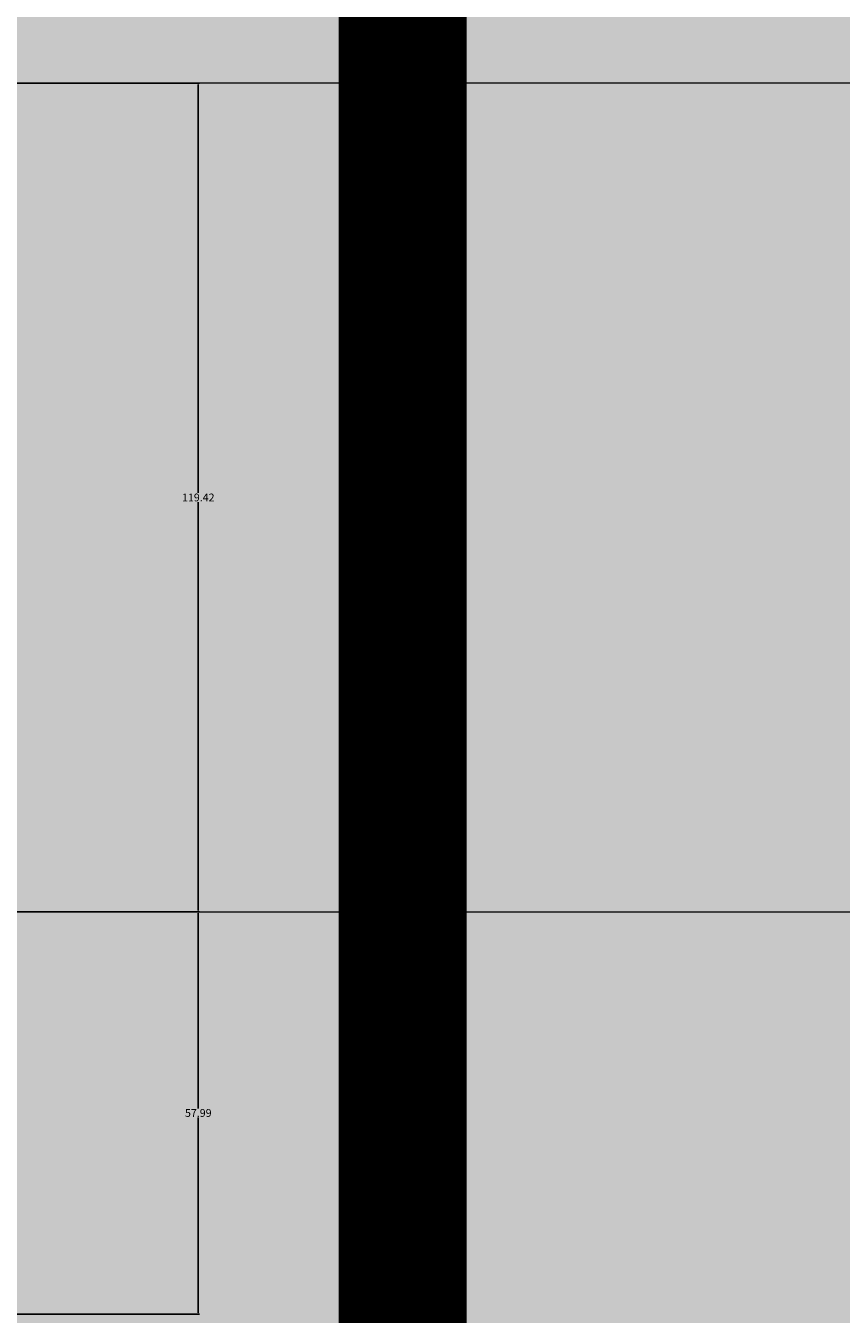
# Model space of a CAD drawing. Units: inches. Extents: x 8 to 634, y 41 to 867.
# Tile 11 of 21: x 297 to 415, y 392 to 577. Entities that reach past the tile are written whole.
import ezdxf

# ---------------------------------------------------------------- set-up
doc = ezdxf.new("R2010")
doc.units = ezdxf.units.IN
doc.header["$MEASUREMENT"] = 0
for name, color, linetype, lineweight in [('A-ANNO-DIMS', 2, 'Continuous', 18), ('A-ELEV-PATT', 252, 'Continuous', 9), ('A-WALL', 7, 'Continuous', 35), ('A-WALL-PANL', 7, 'Continuous', 18), ('A-WALL-PATT', 8, 'Continuous', 9)]:
    doc.layers.add(name, color=color, linetype=linetype, lineweight=lineweight)
doc.styles.get("Standard").update_dxf_attribs({"font": 'arial.ttf'})
doc.dimstyles.get("Standard").update_dxf_attribs({"dimtxt": 1.125, "dimasz": 0.18, "dimexe": 0.18, "dimexo": 0.0625, "dimgap": 0.09, "dimtad": 0, "dimtih": 1, "dimtoh": 1, "dimdec": 4, "dimzin": 0, "dimdsep": 46, "dimlunit": 4, "dimtxsty": 'Standard', "dimcen": 0.09, "dimadec": 0, "dimazin": 0, "dimtfac": 1, "dimtdec": 4, "dimtofl": 0, "dimtmove": 0, "dimatfit": 3, "dimfxl": 1, "dimtolj": 1, "dimtzin": 0, "dimarcsym": 0})

# ---------------------------------------------------------------- blocks, each defined once
blk = doc.blocks.new('*D59')
at = {"layer": 'A-ANNO-DIMS', "color": 0, "lineweight": -2, "transparency": 16777216}
for p, q in [((284.67, 449.75), (322.44, 449.75)), ((322.26, 449.57), (322.26, 421.42)), ((322.26, 391.94), (322.26, 420.09)), ((284.67, 391.76), (322.44, 391.76))]:
    blk.add_line(p, q, dxfattribs=at)
at = {"layer": 'A-ANNO-DIMS', "color": 0, "transparency": 16777216}
for points in [[(322.23, 449.57), (322.29, 449.57), (322.26, 449.75)], [(322.23, 391.94), (322.29, 391.94), (322.26, 391.76)]]:
    blk.add_solid(points, dxfattribs=at)
at = {"layer": 'Defpoints', "color": 0, "transparency": 16777216}
for p in [(284.61, 449.75), (284.61, 391.76), (322.26, 391.76)]:
    blk.add_point(p, dxfattribs=at)
at = {"layer": 'A-ANNO-DIMS', "color": 0, "transparency": 16777216, "insert": (322.26, 420.76), "char_height": 1.125, "attachment_point": 5}
blk.add_mtext('\\A1;57.99', dxfattribs=at)
blk = doc.blocks.new('*D60')
at = {"layer": 'A-ANNO-DIMS', "color": 0, "lineweight": -2, "transparency": 16777216}
for p, q in [((284.67, 569.17), (322.44, 569.17)), ((322.26, 568.99), (322.26, 510.13)), ((322.26, 449.93), (322.26, 508.8)), ((284.67, 449.75), (322.44, 449.75))]:
    blk.add_line(p, q, dxfattribs=at)
at = {"layer": 'A-ANNO-DIMS', "color": 0, "transparency": 16777216}
for points in [[(322.23, 568.99), (322.29, 568.99), (322.26, 569.17)], [(322.23, 449.93), (322.29, 449.93), (322.26, 449.75)]]:
    blk.add_solid(points, dxfattribs=at)
at = {"layer": 'Defpoints', "color": 0, "transparency": 16777216}
for p in [(284.61, 569.17), (284.61, 449.75), (322.26, 449.75)]:
    blk.add_point(p, dxfattribs=at)
at = {"layer": 'A-ANNO-DIMS', "color": 0, "transparency": 16777216, "insert": (322.26, 509.46), "char_height": 1.125, "attachment_point": 5}
blk.add_mtext('\\A1;119.42', dxfattribs=at)

msp = doc.modelspace()

# ---------------------------------------------------------------- hatches: boundary and pattern name
at = {"layer": 'A-ELEV-PATT', "transparency": 33554544}
h = msp.add_hatch(dxfattribs=at)
h.set_pattern_fill('ANSI31', color=256)
h.paths.add_polyline_path([(360.785, 697.6655), (342.6544, 682.1444), (342.6544, 569.1705), (360.785, 569.1705)])
h.paths.add_polyline_path([(360.785, 523.5555), (360.785, 569.1705), (342.6544, 569.1705), (342.6544, 449.7533), (360.785, 449.7533)])
h.paths.add_polyline_path([(360.785, 449.7533), (342.6544, 449.7533), (342.6544, 391.7598), (360.785, 391.7598)])
h.paths.add_polyline_path([(360.785, 391.7598), (342.6544, 391.7598), (342.6544, 272.3426), (360.785, 272.3426)])
h.paths.add_polyline_path([(360.785, 272.3426), (342.6544, 272.3426), (342.6544, 235.5555), (360.785, 235.5555)])
h.paths.add_polyline_path([(360.785, 235.5555), (342.6544, 235.5555), (342.6544, 224.3257), (353.4573, 224.3257), (353.4573, 101.0012), (342.6544, 101.0012), (342.6544, 91.5417), (360.785, 91.5417)])
at = {"layer": 'A-WALL-PATT', "transparency": 33554687}
h = msp.add_hatch(dxfattribs=at)
h.set_pattern_fill('AR-CONC', color=256, scale=3.2)
h.paths.add_polyline_path([(119.7065, 697.6655), (47.3401, 697.6655), (47.3401, 569.1705), (119.7065, 569.1705)])
h.paths.add_polyline_path([(202.1558, 697.6655), (119.7065, 697.6655), (119.7065, 569.1705), (202.1558, 569.1705)])
h.paths.add_polyline_path([(284.6051, 697.6655), (202.1558, 697.6655), (202.1558, 569.1705), (284.6051, 569.1705)])
h.paths.add_polyline_path([(119.7065, 569.1705), (47.3401, 569.1705), (47.3401, 523.5555), (47.3401, 449.7533), (119.7065, 449.7533)])
h.paths.add_polyline_path([(342.6544, 682.1444), (360.785, 697.6655), (284.6051, 697.6655), (284.6051, 569.1705), (342.6544, 569.1705)])
h.paths.add_polyline_path([(342.6544, 569.1705), (284.6051, 569.1705), (284.6051, 449.7533), (342.6544, 449.7533)])
h.paths.add_polyline_path([(418.2881, 691.978), (418.2881, 697.6655), (360.785, 697.6655), (360.785, 569.1705), (418.2881, 569.1705)])
h.paths.add_polyline_path([(418.2881, 569.1705), (360.785, 569.1705), (360.785, 523.5555), (360.785, 449.7533), (418.2881, 449.7533)])
h.paths.add_polyline_path([(594.3501, 697.6655), (539.0002, 697.6655), (539.0002, 691.978), (539.0002, 569.1705), (594.3501, 569.1705)])
h.paths.add_polyline_path([(594.3501, 523.5555), (594.3501, 569.1705), (539.0002, 569.1705), (539.0002, 451.6305), (594.3501, 451.6305)])
h.paths.add_polyline_path([(594.3501, 451.6305), (539.0002, 451.6305), (539.0002, 391.7598), (594.3501, 391.7598)])
h.paths.add_polyline_path([(594.3501, 391.7598), (539.0002, 391.7598), (539.0002, 276.166), (594.3501, 276.166)])
h.paths.add_polyline_path([(418.2881, 449.7533), (360.785, 449.7533), (360.785, 391.7598), (418.2881, 391.7598)])
h.paths.add_polyline_path([(342.6544, 449.7533), (284.6051, 449.7533), (284.6051, 391.7598), (342.6544, 391.7598)])
h.paths.add_polyline_path([(342.6544, 391.7598), (284.6051, 391.7598), (284.6051, 272.3426), (342.6544, 272.3426)])
h.paths.add_polyline_path([(418.2881, 391.7598), (360.785, 391.7598), (360.785, 272.3426), (418.2881, 272.3426)])
h.paths.add_polyline_path([(418.2881, 272.3426), (360.785, 272.3426), (360.785, 235.5555), (418.2881, 235.5555)])
h.paths.add_polyline_path([(342.6544, 272.3426), (284.6051, 272.3426), (284.6051, 235.5555), (295.0049, 235.5555), (342.6544, 235.5555)])
h.paths.add_polyline_path([(594.3501, 276.166), (539.0002, 276.166), (539.0002, 228.4951), (594.3501, 228.4951)])
h.paths.add_polyline_path([(594.3501, 228.4951), (539.0002, 228.4951), (539.0002, 91.5417), (594.3501, 91.5417)])
h.paths.add_polyline_path([(418.2881, 235.5555), (360.785, 235.5555), (360.785, 91.5417), (418.2881, 91.5417)])
h.paths.add_polyline_path([(284.6051, 272.3426), (119.7065, 272.3426), (119.7065, 235.5555), (284.6051, 235.5555)])
h.paths.add_polyline_path([(119.7065, 272.3426), (47.3401, 272.3426), (47.3401, 235.5555), (47.3401, 91.5555), (63.5448, 91.5555), (63.5448, 227.8036), (268.998, 227.8036), (268.998, 91.5555), (295.0049, 91.5555), (295.0049, 222.583), (271.9787, 222.583), (271.9787, 229.0481), (62.4019, 229.0481), (62.4019, 222.583), (61.1827, 222.583), (61.1827, 235.5555), (119.7065, 235.5555)])
h.paths.add_polyline_path([(119.7065, 391.7598), (47.3401, 391.7598), (47.3401, 379.5555), (47.3401, 272.3426), (119.7065, 272.3426)])
h.paths.add_polyline_path([(119.7065, 449.7533), (47.3401, 449.7533), (47.3401, 391.7598), (119.7065, 391.7598)])
h.paths.add_polyline_path([(202.1558, 449.7533), (119.7065, 449.7533), (119.7065, 391.7598), (202.1558, 391.7598)])
h.paths.add_polyline_path([(284.6051, 449.7533), (202.1558, 449.7533), (202.1558, 391.7598), (284.6051, 391.7598)])

# ---------------------------------------------------------------- linework, layer by layer
at = {"layer": 'A-WALL'}
for p, q in [((360.785, 523.5555), (360.785, 697.6655)), ((342.6544, 682.1444), (342.6544, 91.5555)), ((360.785, 235.5555), (360.785, 523.5555))]:
    msp.add_line(p, q, dxfattribs=at)
at = {"layer": 'A-WALL-PANL'}
for p, q in [((418.2881, 569.1705), (47.3401, 569.1705)), ((284.6051, 449.7533), (418.2881, 449.7533))]:
    msp.add_line(p, q, dxfattribs=at)

# ---------------------------------------------------------------- dimensions: what is measured, and where the dimension line sits
at = {"layer": 'A-ANNO-DIMS'}
for base, p1, p2, picture, middle in [((322.2551, 449.7533), (284.6051, 569.1705), (284.6051, 449.7533), '*D60', (322.2551, 509.4619)), ((322.2551, 391.7598), (284.6051, 449.7533), (284.6051, 391.7598), '*D59', (322.2551, 420.7566))]:
    dim = msp.add_linear_dim(base=base, p1=p1, p2=p2, angle=270, dimstyle='Standard', override={"dimdec": 2, "dimlfac": 1, "dimrnd": 0, "dimzin": 0, "dimdsep": 46, "dimlunit": 2}, dxfattribs=at)
    dim.commit()
    dim.dimension.update_dxf_attribs({"geometry": picture, "text_midpoint": middle})

doc.saveas('drawing.dxf')
